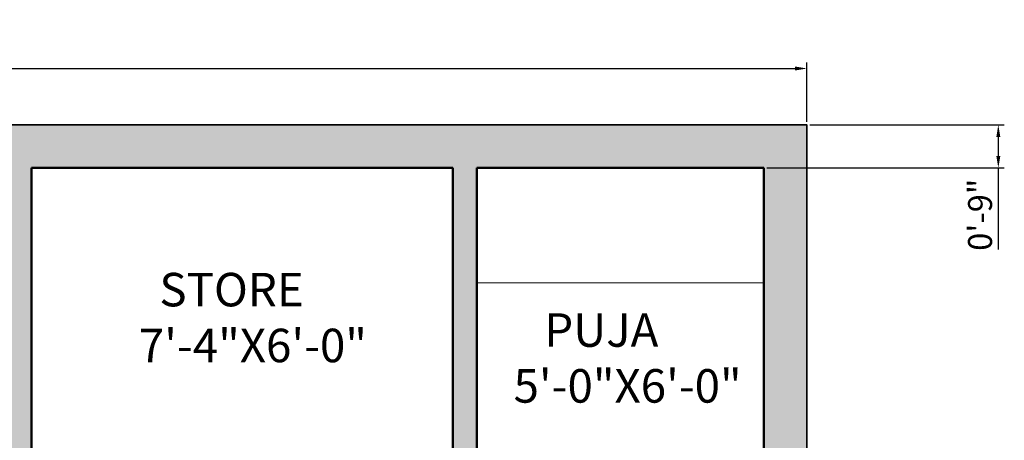
# Model space of a CAD drawing. Units: inches. Extents: x 1734 to 4011, y 1071 to 1891.
# Tile 23 of 27: x 3311 to 3517, y 1766 to 1854. Entities that reach past the tile are written whole.
import ezdxf

# ---------------------------------------------------------------- set-up
doc = ezdxf.new("R2010")
doc.units = ezdxf.units.IN
for name, color, linetype, lineweight in [('A-ANNO-DIMS', 2, 'Continuous', 18), ('A-AREA-IDEN', 3, 'Continuous', 18), ('A-FURN', 8, 'Continuous', 18), ('A-WALL', 7, 'Continuous', 50), ('A-WALL-PATT', 8, 'Continuous', 13), ('C-PROP', 1, 'Continuous', 35)]:
    doc.layers.add(name, color=color, linetype=linetype, lineweight=lineweight)
doc.styles.get("Standard").update_dxf_attribs({"font": 'arial.ttf'})
doc.dimstyles.new('ISO-25', dxfattribs={"dimtxt": 5, "dimasz": 2.5, "dimexe": 1.25, "dimexo": 0.625, "dimtad": 1, "dimdec": 1, "dimlunit": 3, "dimtxsty": 'Standard', "dimcen": 2.5, "dimclrt": 1, "dimadec": 0, "dimazin": 0, "dimtfac": 1, "dimtdec": 1, "dimtmove": 0, "dimatfit": 3, "dimfxl": 1, "dimarcsym": 0})

# ---------------------------------------------------------------- blocks, each defined once
blk = doc.blocks.new('*D70')
at = {"layer": 'A-ANNO-DIMS', "color": 0, "lineweight": -2, "transparency": 16777216}
for p, q in [((3115.99, 1832.44), (3115.99, 1844.85)), ((3118.49, 1843.6), (3473.49, 1843.6)), ((3475.99, 1832.44), (3475.99, 1844.85))]:
    blk.add_line(p, q, dxfattribs=at)
at = {"layer": 'A-ANNO-DIMS', "color": 0, "transparency": 16777216}
for points in [[(3118.49, 1844.02), (3118.49, 1843.18), (3115.99, 1843.6)], [(3473.49, 1844.02), (3473.49, 1843.18), (3475.99, 1843.6)]]:
    blk.add_solid(points, dxfattribs=at)
at = {"layer": 'Defpoints', "color": 0, "transparency": 16777216}
for p in [(3475.99, 1843.6), (3115.99, 1831.82), (3475.99, 1831.82)]:
    blk.add_point(p, dxfattribs=at)
at = {"layer": 'A-ANNO-DIMS', "color": 0, "transparency": 16777216, "insert": (3295.99, 1848.82), "char_height": 5, "attachment_point": 5}
blk.add_mtext("{\\H1.8x;30'}", dxfattribs=at)
blk = doc.blocks.new('*D120')
at = {"layer": 'A-ANNO-DIMS', "color": 0, "lineweight": -2, "transparency": 16777216}
for p, q in [((3476.62, 1831.82), (3517.24, 1831.82)), ((3515.99, 1829.32), (3515.99, 1825.32)), ((3467.62, 1822.82), (3517.24, 1822.82)), ((3515.99, 1822.82), (3515.99, 1805.78))]:
    blk.add_line(p, q, dxfattribs=at)
at = {"layer": 'A-ANNO-DIMS', "color": 0, "transparency": 16777216}
for points in [[(3515.58, 1829.32), (3516.41, 1829.32), (3515.99, 1831.82)], [(3515.58, 1825.32), (3516.41, 1825.32), (3515.99, 1822.82)]]:
    blk.add_solid(points, dxfattribs=at)
at = {"layer": 'Defpoints', "color": 0, "transparency": 16777216}
for p in [(3475.99, 1831.82), (3466.99, 1822.82), (3515.99, 1822.82)]:
    blk.add_point(p, dxfattribs=at)
at = {"layer": 'A-ANNO-DIMS', "color": 1, "transparency": 16777216, "insert": (3512.82, 1813.05), "char_height": 5, "attachment_point": 5, "rotation": 90}
blk.add_mtext('0\'-9"', dxfattribs=at)

msp = doc.modelspace()

# ---------------------------------------------------------------- hatches: boundary and pattern name
at = {"layer": 'A-WALL-PATT'}
h = msp.add_hatch(color=256, dxfattribs=at)
h.dxf.hatch_style = 1
h.paths.add_polyline_path([(3475.99, 1831.82), (3115.99, 1831.82), (3115.99, 1745.82), (3130.99, 1745.82), (3130.99, 1750.82), (3124.99, 1750.82), (3124.99, 1822.82), (3214.99, 1822.82), (3214.99, 1780.82), (3219.99, 1780.82), (3219.99, 1822.82), (3308.99, 1822.82), (3308.99, 1750.82), (3254.99, 1750.82), (3254.99, 1745.82), (3308.99, 1745.82), (3308.99, 1604.82), (3313.99, 1604.82), (3313.99, 1745.82), (3366.99, 1745.82), (3366.99, 1750.82), (3313.99, 1750.82), (3313.99, 1822.82), (3401.99, 1822.82), (3401.99, 1750.82), (3396.99, 1750.82), (3396.99, 1745.82), (3411.99, 1745.82), (3411.99, 1750.82), (3406.99, 1750.82), (3406.99, 1822.82), (3466.99, 1822.82), (3466.99, 1750.82), (3441.99, 1750.82), (3441.99, 1745.82), (3466.99, 1745.82), (3466.99, 1517.82), (3452.49, 1517.82), (3452.49, 1512.82), (3466.99, 1512.82), (3466.99, 1458.82), (3446.49, 1458.82), (3446.49, 1453.82), (3466.99, 1453.82), (3466.99, 1237.82), (3372.99, 1237.82), (3372.99, 1228.82), (3466.99, 1228.82), (3466.99, 1120.82), (3309.99, 1120.82), (3309.99, 1184.82), (3310.99, 1184.82), (3310.99, 1189.82), (3303.99, 1189.82), (3303.99, 1120.82), (3291.99, 1120.82), (3291.99, 1111.82), (3475.99, 1111.82)])
h.paths.add_polyline_path([(3169.99, 1745.82), (3224.99, 1745.82), (3224.99, 1750.82), (3154.99, 1750.82), (3154.99, 1745.82), (3160.99, 1745.82), (3160.99, 1636.82), (3169.99, 1636.82)], flags=17)
h.paths.add_polyline_path([(3169.99, 1588.82), (3160.99, 1588.82), (3160.99, 1559.82), (3313.99, 1559.82), (3313.99, 1568.82), (3308.99, 1568.82), (3308.99, 1564.82), (3169.99, 1564.82)], flags=17)
h.paths.add_polyline_path([(3416.49, 1517.82), (3401.99, 1517.82), (3401.99, 1512.82), (3416.49, 1512.82)], flags=17)
h.paths.add_polyline_path([(3371.99, 1517.82), (3366.99, 1517.82), (3366.99, 1453.82), (3392.49, 1453.82), (3392.49, 1458.82), (3371.99, 1458.82)], flags=17)
h.paths.add_polyline_path([(3258.99, 1529.82), (3160.99, 1529.82), (3160.99, 1494.82), (3169.99, 1494.82), (3169.99, 1524.82), (3253.99, 1524.82), (3253.99, 1520.82), (3258.99, 1520.82)], flags=17)
h.paths.add_polyline_path([(3263.99, 1458.82), (3258.99, 1458.82), (3258.99, 1490.82), (3253.99, 1490.82), (3253.99, 1458.82), (3169.99, 1458.82), (3169.99, 1470.82), (3160.99, 1470.82), (3160.99, 1387.82), (3169.99, 1387.82), (3169.99, 1453.82), (3263.99, 1453.82)], flags=17)
h.paths.add_polyline_path([(3313.99, 1453.82), (3318.99, 1453.82), (3318.99, 1458.82), (3299.99, 1458.82), (3299.99, 1453.82), (3308.99, 1453.82), (3308.99, 1321.82), (3266.49, 1321.82), (3266.49, 1312.82), (3313.99, 1312.82)], flags=17)
h.paths.add_polyline_path([(3212.49, 1321.82), (3169.99, 1321.82), (3169.99, 1339.82), (3160.99, 1339.82), (3160.99, 1312.82), (3212.49, 1312.82)], flags=17)
h.paths.add_polyline_path([(3313.99, 1288.82), (3304.99, 1288.82), (3304.99, 1285.82), (3313.99, 1285.82)], flags=17)
h.paths.add_polyline_path([(3324.99, 1237.82), (3304.99, 1237.82), (3304.99, 1228.82), (3324.99, 1228.82)], flags=17)

# ---------------------------------------------------------------- linework, layer by layer
at = {"layer": 'A-FURN'}
msp.add_line((3406.99, 1798.82), (3466.99, 1798.82), dxfattribs=at)
at = {"layer": 'A-WALL'}
for p, q in [((3313.99, 1822.82), (3401.99, 1822.82)), ((3313.99, 1750.82), (3313.99, 1822.82)), ((3401.99, 1750.82), (3401.99, 1822.82)), ((3406.99, 1822.82), (3466.99, 1822.82)), ((3406.99, 1750.82), (3406.99, 1822.82)), ((3466.99, 1822.82), (3466.99, 1750.82))]:
    msp.add_line(p, q, dxfattribs=at)
at = {"layer": 'C-PROP'}
msp.add_lwpolyline([(3171.99, 1111.82), (3115.99, 1111.82), (3115.99, 1831.82), (3475.99, 1831.82), (3475.99, 1111.82), (3291.99, 1111.82)], dxfattribs=at)

# ---------------------------------------------------------------- texts
at = {"layer": 'A-AREA-IDEN', "char_height": 7, "attachment_point": 1}
for s, insert in [('  STORE\\P7\'-4"X6\'-0"', (3336.4, 1800.91)), ('   PUJA\\P5\'-0"X6\'-0"', (3414.7, 1792.47))]:
    msp.add_mtext_dynamic_manual_height_columns(s, width=86.9528, gutter_width=12.5, heights=[18.94], dxfattribs=dict(at, insert=insert))

# ---------------------------------------------------------------- dimensions: what is measured, and where the dimension line sits
at = {"layer": 'A-ANNO-DIMS'}
dim = msp.add_linear_dim(base=(3475.99, 1843.6), p1=(3115.99, 1831.82), p2=(3475.99, 1831.82), text='{\\H1.8x;<>}', dimstyle='ISO-25', override={"dimclrd": 0, "dimclre": 0, "dimclrt": 0}, dxfattribs=at)
dim.commit()
dim.dimension.update_dxf_attribs({"geometry": '*D70', "text_midpoint": (3295.99, 1848.82)})
dim = msp.add_linear_dim(base=(3515.99, 1822.82), p1=(3475.99, 1831.82), p2=(3466.99, 1822.82), angle=90, dimstyle='ISO-25', override={"dimdec": 1, "dimlfac": 1, "dimrnd": 0, "dimzin": 1, "dimdsep": 46, "dimlunit": 4, "dimfrac": 2}, dxfattribs=at)
dim.commit()
dim.dimension.update_dxf_attribs({"geometry": '*D120', "text_midpoint": (3512.82, 1813.05)})

doc.saveas('drawing.dxf')
